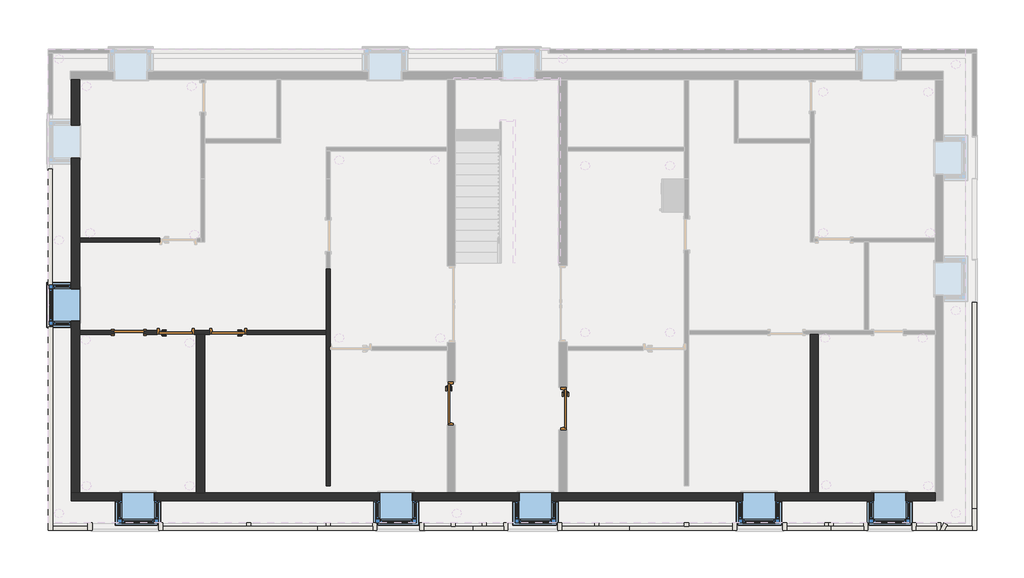
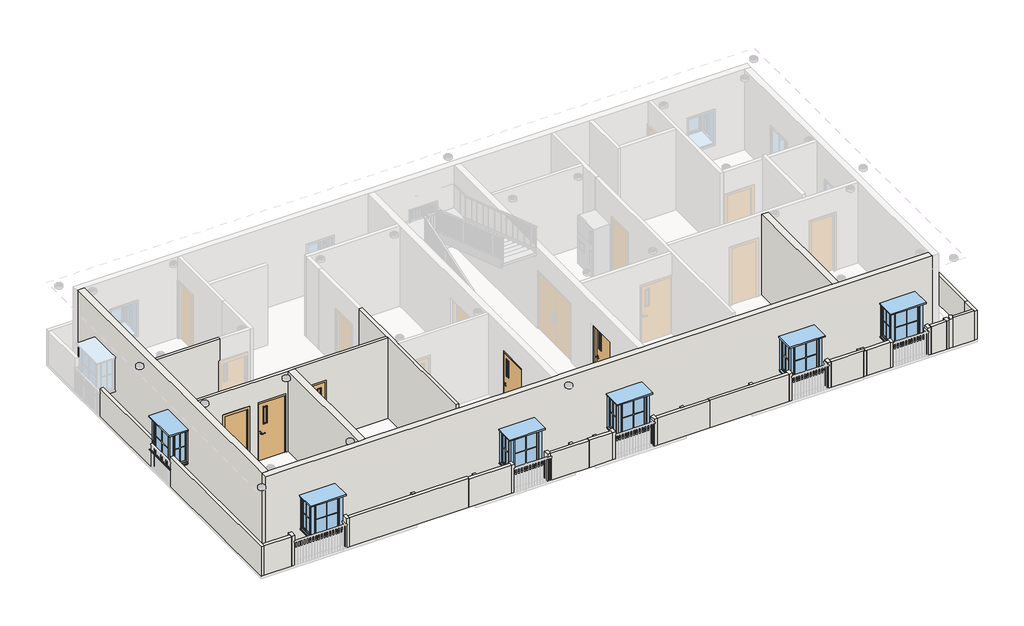
# One storey, part 1 of 7: 42 walls, 6 windows, 5 doors.
# Revit data of these elements (continued)
# Element 43 (IfcWall, "Generic - 4.5\"") (continued)
#   wall height = 3' - 6.78233"
#   Phase Created = New Construction
#   Base Constraint = 1 STH FLOOR
#   Top Constraint = 2 ND FLOOR
#   Materials on its faces: "Default Wall"
# Elements 44, 45, 46, 47 (IfcWall, "Generic - 9\"")
#   Top Offset = -0' - 6"
#   Base Offset = 0' - 0"
#   wall height = 10' - 0"
#   Phase Created = New Construction
#   Base Constraint = 1 STH FLOOR
#   Top Constraint = 2 ND FLOOR
#   Materials on its faces: "Concrete Masonry Units"
# Element 48 (IfcWindow, "Window-Bay-Casement-Box-90_Degree_Angle-Center_Fixed : 4'X3'")
#   Mark = "110"
#   Interior Trim Visibility = yes
#   Exterior Trim Visibility = yes
#   Phase Created = New Construction
#   Materials on its faces: "Clad - White", "Wood - Stained", "Glass"
# Element 49 (IfcWindow, "Window-Bay-Casement-Box-90_Degree_Angle-Center_Fixed : 4'X3'")
#   Mark = "111"
#   Interior Trim Visibility = yes
#   Exterior Trim Visibility = yes
#   Phase Created = New Construction
#   Materials on its faces: "Clad - White", "Wood - Stained", "Glass"
# Element 50 (IfcWindow, "Window-Bay-Casement-Box-90_Degree_Angle-Center_Fixed : 4'X3'")
#   Mark = "112"
#   Interior Trim Visibility = yes
#   Exterior Trim Visibility = yes
#   Phase Created = New Construction
#   Materials on its faces: "Clad - White", "Wood - Stained", "Glass"
# Element 51 (IfcWindow, "Window-Bay-Casement-Box-90_Degree_Angle-Center_Fixed : 4'X3'")
#   Mark = "113"
#   Interior Trim Visibility = yes
#   Exterior Trim Visibility = yes
#   Phase Created = New Construction
#   Materials on its faces: "Clad - White", "Wood - Stained", "Glass"
# Element 52 (IfcWindow, "Window-Bay-Casement-Box-90_Degree_Angle-Center_Fixed : 4'X3'")
#   Mark = "114"
#   Interior Trim Visibility = yes
#   Exterior Trim Visibility = yes
#   Phase Created = New Construction
#   Materials on its faces: "Clad - White", "Wood - Stained", "Glass"
# Element 53 (IfcWindow, "Window-Bay-Casement-Box-90_Degree_Angle-Center_Fixed : 4'X3'")
#   Mark = "117"
#   Interior Trim Visibility = yes
#   Exterior Trim Visibility = yes
#   Phase Created = New Construction
#   Materials on its faces: "Clad - White", "Wood - Stained", "Glass"
# Materials
#   "Wood - Birch": class "Wood", colour RGB 166 116 52, transparency 0, Cost = 0
#   "Glass": class "Glass", colour RGB 0 128 192, transparency 0.75, Description = "Soda Lime Glass", Cost = 0
#   "Metal - Paint Finish - Grey": class "Paint", colour RGB 104 104 104, transparency 0, Cost = 0
#   "Aluminum": class "Metal", colour RGB 247 247 247, transparency 0, Description = "Aluminum 6061", Cost = 0
#   "Door - Panel": class "Wood", colour RGB 210 159 95, transparency 0, Cost = 0
#   "Door - Frame": colour RGB 118 70 51, transparency 0, Cost = 0
#   "Concrete Masonry Units": class "Masonry", colour RGB 227 227 227, transparency 0, Description = "Concrete masonry units", Cost = 0
#   "Wood - Stained": class "Wood", colour RGB 224 178 126, transparency 0, Cost = 0
#   "Clad - White": class "Wood", colour RGB 242 242 238, transparency 0, Cost = 0
#   "Default Wall": colour RGB 128 128 128, transparency 0, Cost = 0
